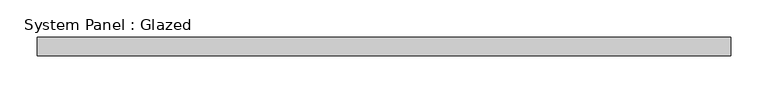
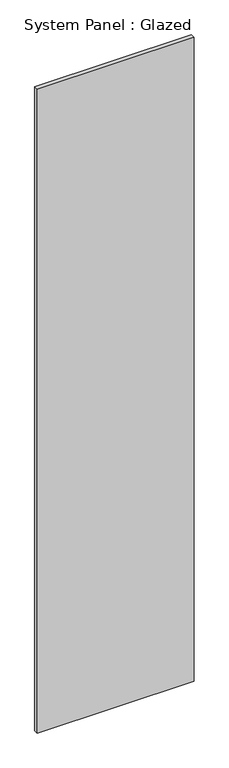
"""IFC4 building model written with IfcOpenShell, lengths in millimetres: plate geometry, System Panel : Glazed."""

from ifc_helpers import new_model, si_unit, origin, origin_with_axes, place, context, project, spatial, polyline, outline, extrude, source, transform, mapped, element, save


def system_panel_glazed_6cc658bf(model_context):
    return source(origin(), model_context, "Body", "SweptSolid", [
        extrude(outline(polyline([(467.7358042, 19.05), (-467.7358042, 19.05), (-467.7358042, 44.45), (467.7358042, 44.45), (467.7358042, 19.05)])), origin_with_axes(), (0.0, 0.0, 1.0), 4056.7935364),
    ])


if __name__ == "__main__":
    model = new_model("IFC4")
    model_context = context("Model", 3, world=origin())
    ifc_project = project(units=[si_unit("LENGTHUNIT", "METRE", prefix="MILLI")], contexts=[model_context])
    site = spatial("IfcSite", under=ifc_project)
    building = spatial("IfcBuilding", under=site)
    placement = place(None, origin())
    system_panel_glazed_shape = system_panel_glazed_6cc658bf(model_context)
    element("IfcPlate", 1, ObjectType="System Panel : Glazed", at=placement, inside=building, context=model_context, shape_type="MappedRepresentation", body=[
        mapped(system_panel_glazed_shape, transform((0.0, 0.0, 0.0), x_axis=(1.0, 0.0, 0.0), y_axis=(0.0, 1.0, 0.0), z_axis=(0.0, 0.0, 1.0))),
    ])
    save(model, "model.ifc")

# Revit data of these elements
# Type "System Panel : Glazed"
#   Construction Type Id = "GSP4R"
#   Analytic Construction = "1/8 in Pilkington single glazing"
#   Visual Light Transmittance = 0.9
#   Solar Heat Gain Coefficient = 0.86
#   Heat Transfer Coefficient (U) = 1.18115 BTU/(h·ft²·°F)
#   Define Thermal Properties by = 1
# Element 1 (IfcPlate, "System Panel : Glazed")
#   Materials on its faces: "Glass"
# Materials
#   "Glass": class "Glass", colour RGB 0 128 192, transparency 0.75, Description = "Soda Lime Glass", Cost = 0
